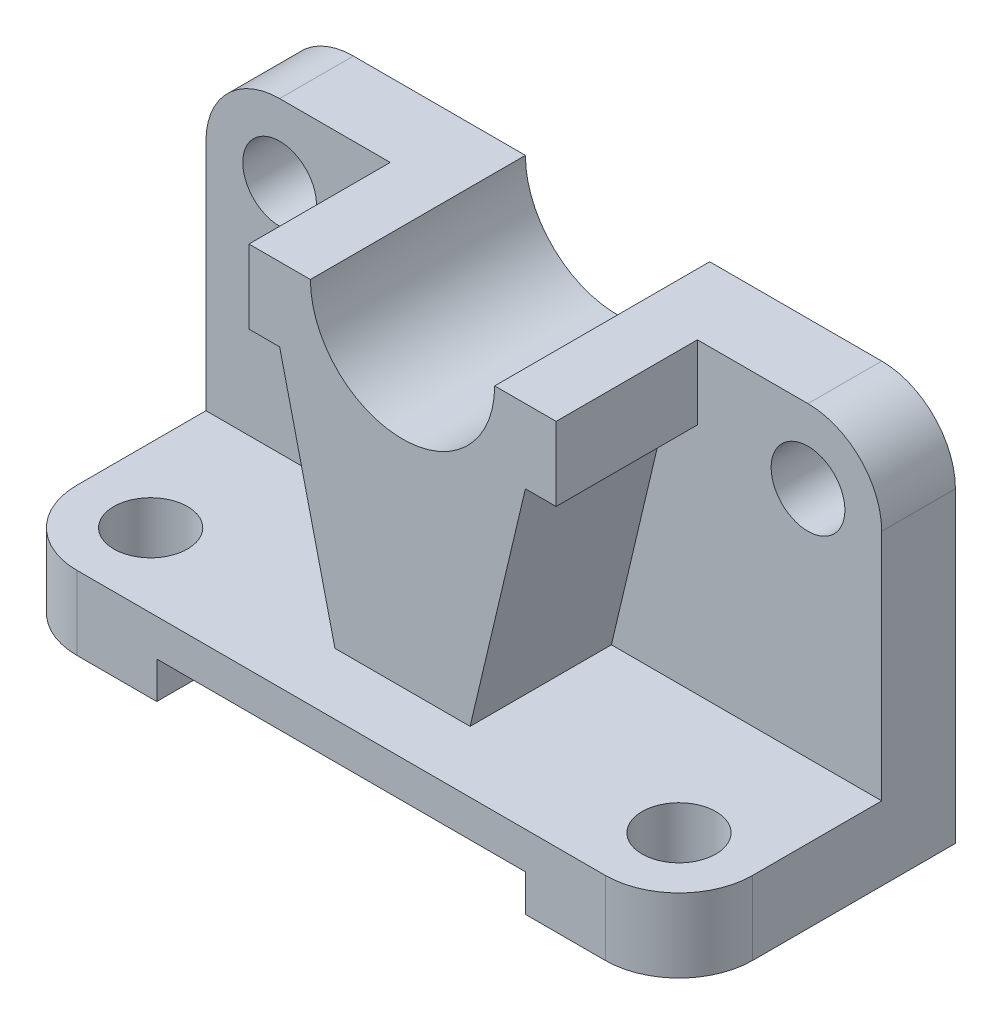
ISO-10303-21;
HEADER;
FILE_DESCRIPTION(('STEP AP214'),'2;1');
FILE_NAME('part.step','',(''),(''),'','','');
FILE_SCHEMA(('AUTOMOTIVE_DESIGN { 1 0 10303 214 1 1 1 1 }'));
ENDSEC;
DATA;
#1=APPLICATION_CONTEXT('core data for automotive mechanical design processes');
#2=APPLICATION_PROTOCOL_DEFINITION('international standard','automotive_design',2000,#1);
#3=PRODUCT_CONTEXT('',#1,'mechanical');
#4=PRODUCT('Part','Part','',(#3));
#5=PRODUCT_RELATED_PRODUCT_CATEGORY('part','',(#4));
#6=PRODUCT_DEFINITION_FORMATION('','',#4);
#7=PRODUCT_DEFINITION_CONTEXT('part definition',#1,'design');
#8=PRODUCT_DEFINITION('design','',#6,#7);
#9=PRODUCT_DEFINITION_SHAPE('','',#8);
#10=(LENGTH_UNIT() NAMED_UNIT(*) SI_UNIT(.MILLI.,.METRE.));
#11=(NAMED_UNIT(*) PLANE_ANGLE_UNIT() SI_UNIT($,.RADIAN.));
#12=(NAMED_UNIT(*) SI_UNIT($,.STERADIAN.) SOLID_ANGLE_UNIT());
#13=UNCERTAINTY_MEASURE_WITH_UNIT(LENGTH_MEASURE(1.E-05),#10,'distance_accuracy_value','');
#14=(GEOMETRIC_REPRESENTATION_CONTEXT(3) GLOBAL_UNCERTAINTY_ASSIGNED_CONTEXT((#13)) GLOBAL_UNIT_ASSIGNED_CONTEXT((#10,
#11,#12)) REPRESENTATION_CONTEXT('',''));
#15=CARTESIAN_POINT('',(0.,0.,0.));
#16=DIRECTION('',(0.,0.,1.));
#17=DIRECTION('',(1.,0.,0.));
#18=AXIS2_PLACEMENT_3D('',#15,#16,#17);
#19=CARTESIAN_POINT('',(43.,50.,-10.5));
#20=DIRECTION('',(0.,0.,1.));
#21=DIRECTION('',(1.,0.,0.));
#22=AXIS2_PLACEMENT_3D('',#19,#20,#21);
#23=PLANE('',#22);
#24=CARTESIAN_POINT('',(-43.,50.,-10.5));
#25=DIRECTION('',(0.,0.,-1.));
#26=DIRECTION('',(-1.,0.,0.));
#27=AXIS2_PLACEMENT_3D('',#24,#25,#26);
#28=CIRCLE('',#27,5.99999999999999);
#29=CARTESIAN_POINT('',(-49.,50.,-10.5));
#30=VERTEX_POINT('',#29);
#31=EDGE_CURVE('E298',#30,#30,#28,.T.);
#32=ORIENTED_EDGE('',*,*,#31,.T.);
#33=EDGE_LOOP('',(#32));
#34=FACE_BOUND('',#33,.T.);
#35=DIRECTION('',(1.,0.,0.));
#36=VECTOR('',#35,1.);
#37=CARTESIAN_POINT('',(-43.,12.,-10.5));
#38=LINE('',#37,#36);
#39=CARTESIAN_POINT('',(-55.,12.,-10.5));
#40=VERTEX_POINT('',#39);
#41=CARTESIAN_POINT('',(-11.,12.,-10.5));
#42=VERTEX_POINT('',#41);
#43=EDGE_CURVE('E347',#40,#42,#38,.T.);
#44=ORIENTED_EDGE('',*,*,#43,.T.);
#45=DIRECTION('',(0.230466383879213,-0.973080287490009,0.));
#46=VECTOR('',#45,1.);
#47=CARTESIAN_POINT('',(-7.72459016393442,-1.82950819672131,-10.5));
#48=LINE('',#47,#46);
#49=CARTESIAN_POINT('',(-20.,50.,-10.5));
#50=VERTEX_POINT('',#49);
#51=EDGE_CURVE('E245',#50,#42,#48,.T.);
#52=ORIENTED_EDGE('',*,*,#51,.F.);
#53=DIRECTION('',(-1.,0.,0.));
#54=VECTOR('',#53,1.);
#55=CARTESIAN_POINT('',(0.,50.,-10.5));
#56=LINE('',#55,#54);
#57=CARTESIAN_POINT('',(-25.,50.,-10.5));
#58=VERTEX_POINT('',#57);
#59=EDGE_CURVE('E250',#50,#58,#56,.T.);
#60=ORIENTED_EDGE('',*,*,#59,.T.);
#61=DIRECTION('',(0.,-1.,0.));
#62=VECTOR('',#61,1.);
#63=CARTESIAN_POINT('',(-25.,50.,-10.5));
#64=LINE('',#63,#62);
#65=CARTESIAN_POINT('',(-25.,62.,-10.5));
#66=VERTEX_POINT('',#65);
#67=EDGE_CURVE('E11',#66,#58,#64,.T.);
#68=ORIENTED_EDGE('',*,*,#67,.F.);
#69=DIRECTION('',(1.,0.,0.));
#70=VECTOR('',#69,1.);
#71=CARTESIAN_POINT('',(42.9999999999999,62.,-10.5));
#72=LINE('',#71,#70);
#73=CARTESIAN_POINT('',(-42.9999999999999,62.,-10.5));
#74=VERTEX_POINT('',#73);
#75=EDGE_CURVE('E321',#74,#66,#72,.T.);
#76=ORIENTED_EDGE('',*,*,#75,.F.);
#77=CARTESIAN_POINT('',(-43.,50.,-10.5));
#78=DIRECTION('',(0.,0.,-1.));
#79=DIRECTION('',(1.,0.,0.));
#80=AXIS2_PLACEMENT_3D('',#77,#78,#79);
#81=CIRCLE('',#80,12.);
#82=CARTESIAN_POINT('',(-55.,49.9999999999999,-10.5));
#83=VERTEX_POINT('',#82);
#84=EDGE_CURVE('E320',#83,#74,#81,.T.);
#85=ORIENTED_EDGE('',*,*,#84,.F.);
#86=DIRECTION('',(0.,1.,0.));
#87=VECTOR('',#86,1.);
#88=CARTESIAN_POINT('',(-55.,0.,-10.5));
#89=LINE('',#88,#87);
#90=EDGE_CURVE('E314',#40,#83,#89,.T.);
#91=ORIENTED_EDGE('',*,*,#90,.F.);
#92=EDGE_LOOP('',(#44,#52,#60,#68,#76,#85,#91));
#93=FACE_BOUND('',#92,.T.);
#94=ADVANCED_FACE('F50',(#34,#93),#23,.T.);
#95=DIRECTION('',(-0.230466383879213,-0.97308028749001,0.));
#96=VECTOR('',#95,1.);
#97=CARTESIAN_POINT('',(7.72459016393442,-1.82950819672131,-10.5));
#98=LINE('',#97,#96);
#99=CARTESIAN_POINT('',(20.,50.,-10.5));
#100=VERTEX_POINT('',#99);
#101=CARTESIAN_POINT('',(11.,12.,-10.5));
#102=VERTEX_POINT('',#101);
#103=EDGE_CURVE('E260',#100,#102,#98,.T.);
#104=ORIENTED_EDGE('',*,*,#103,.T.);
#105=CARTESIAN_POINT('',(55.,12.,-10.5));
#106=VERTEX_POINT('',#105);
#107=EDGE_CURVE('E339',#102,#106,#38,.T.);
#108=ORIENTED_EDGE('',*,*,#107,.T.);
#109=DIRECTION('',(0.,-1.,0.));
#110=VECTOR('',#109,1.);
#111=CARTESIAN_POINT('',(55.,0.,-10.5));
#112=LINE('',#111,#110);
#113=CARTESIAN_POINT('',(55.,49.9999999999999,-10.5));
#114=VERTEX_POINT('',#113);
#115=EDGE_CURVE('E313',#114,#106,#112,.T.);
#116=ORIENTED_EDGE('',*,*,#115,.F.);
#117=CARTESIAN_POINT('',(43.,50.,-10.5));
#118=DIRECTION('',(0.,0.,-1.));
#119=DIRECTION('',(1.,0.,0.));
#120=AXIS2_PLACEMENT_3D('',#117,#118,#119);
#121=CIRCLE('',#120,12.);
#122=CARTESIAN_POINT('',(42.9999999999999,62.,-10.5));
#123=VERTEX_POINT('',#122);
#124=EDGE_CURVE('E322',#123,#114,#121,.T.);
#125=ORIENTED_EDGE('',*,*,#124,.F.);
#126=CARTESIAN_POINT('',(25.,62.,-10.5));
#127=VERTEX_POINT('',#126);
#128=EDGE_CURVE('E319',#127,#123,#72,.T.);
#129=ORIENTED_EDGE('',*,*,#128,.F.);
#130=DIRECTION('',(0.,-1.,0.));
#131=VECTOR('',#130,1.);
#132=CARTESIAN_POINT('',(25.,50.,-10.5));
#133=LINE('',#132,#131);
#134=CARTESIAN_POINT('',(25.,50.,-10.5));
#135=VERTEX_POINT('',#134);
#136=EDGE_CURVE('E218',#127,#135,#133,.T.);
#137=ORIENTED_EDGE('',*,*,#136,.T.);
#138=DIRECTION('',(1.,0.,0.));
#139=VECTOR('',#138,1.);
#140=CARTESIAN_POINT('',(0.,50.,-10.5));
#141=LINE('',#140,#139);
#142=EDGE_CURVE('E62',#100,#135,#141,.T.);
#143=ORIENTED_EDGE('',*,*,#142,.F.);
#144=EDGE_LOOP('',(#104,#108,#116,#125,#129,#137,#143));
#145=FACE_BOUND('',#144,.T.);
#146=CARTESIAN_POINT('',(43.,50.,-10.5));
#147=DIRECTION('',(0.,0.,-1.));
#148=DIRECTION('',(-1.,0.,0.));
#149=AXIS2_PLACEMENT_3D('',#146,#147,#148);
#150=CIRCLE('',#149,5.99999999999999);
#151=CARTESIAN_POINT('',(37.,50.,-10.5));
#152=VERTEX_POINT('',#151);
#153=EDGE_CURVE('E304',#152,#152,#150,.T.);
#154=ORIENTED_EDGE('',*,*,#153,.T.);
#155=EDGE_LOOP('',(#154));
#156=FACE_BOUND('',#155,.T.);
#157=ADVANCED_FACE('F454',(#145,#156),#23,.T.);
#158=CARTESIAN_POINT('',(0.,62.,12.5));
#159=DIRECTION('',(0.,0.,-1.));
#160=DIRECTION('',(-1.,0.,0.));
#161=AXIS2_PLACEMENT_3D('',#158,#159,#160);
#162=PLANE('',#161);
#163=DIRECTION('',(1.,0.,0.));
#164=VECTOR('',#163,1.);
#165=CARTESIAN_POINT('',(0.,50.,12.5));
#166=LINE('',#165,#164);
#167=CARTESIAN_POINT('',(-25.,50.,12.5));
#168=VERTEX_POINT('',#167);
#169=CARTESIAN_POINT('',(-20.,50.,12.5));
#170=VERTEX_POINT('',#169);
#171=EDGE_CURVE('E253',#168,#170,#166,.T.);
#172=ORIENTED_EDGE('',*,*,#171,.T.);
#173=DIRECTION('',(-0.230466383879213,0.97308028749001,0.));
#174=VECTOR('',#173,1.);
#175=CARTESIAN_POINT('',(-7.72459016393442,-1.82950819672131,12.5));
#176=LINE('',#175,#174);
#177=CARTESIAN_POINT('',(-11.,12.,12.5));
#178=VERTEX_POINT('',#177);
#179=EDGE_CURVE('E251',#178,#170,#176,.T.);
#180=ORIENTED_EDGE('',*,*,#179,.F.);
#181=DIRECTION('',(1.,0.,0.));
#182=VECTOR('',#181,1.);
#183=CARTESIAN_POINT('',(0.,12.,12.5));
#184=LINE('',#183,#182);
#185=CARTESIAN_POINT('',(11.,12.,12.5));
#186=VERTEX_POINT('',#185);
#187=EDGE_CURVE('E227',#178,#186,#184,.T.);
#188=ORIENTED_EDGE('',*,*,#187,.T.);
#189=DIRECTION('',(0.230466383879213,0.973080287490009,0.));
#190=VECTOR('',#189,1.);
#191=CARTESIAN_POINT('',(7.72459016393442,-1.82950819672131,12.5));
#192=LINE('',#191,#190);
#193=CARTESIAN_POINT('',(20.,50.,12.5));
#194=VERTEX_POINT('',#193);
#195=EDGE_CURVE('E217',#186,#194,#192,.T.);
#196=ORIENTED_EDGE('',*,*,#195,.T.);
#197=DIRECTION('',(-1.,0.,0.));
#198=VECTOR('',#197,1.);
#199=CARTESIAN_POINT('',(0.,50.,12.5));
#200=LINE('',#199,#198);
#201=CARTESIAN_POINT('',(25.,50.,12.5));
#202=VERTEX_POINT('',#201);
#203=EDGE_CURVE('E211',#202,#194,#200,.T.);
#204=ORIENTED_EDGE('',*,*,#203,.F.);
#205=DIRECTION('',(0.,-1.,0.));
#206=VECTOR('',#205,1.);
#207=CARTESIAN_POINT('',(25.,0.,12.5));
#208=LINE('',#207,#206);
#209=CARTESIAN_POINT('',(25.,62.,12.5));
#210=VERTEX_POINT('',#209);
#211=EDGE_CURVE('E216',#210,#202,#208,.T.);
#212=ORIENTED_EDGE('',*,*,#211,.F.);
#213=DIRECTION('',(1.,0.,0.));
#214=VECTOR('',#213,1.);
#215=CARTESIAN_POINT('',(25.,62.,12.5));
#216=LINE('',#215,#214);
#217=CARTESIAN_POINT('',(15.,62.,12.5));
#218=VERTEX_POINT('',#217);
#219=EDGE_CURVE('E264',#218,#210,#216,.T.);
#220=ORIENTED_EDGE('',*,*,#219,.F.);
#221=CARTESIAN_POINT('',(0.,62.,12.5));
#222=DIRECTION('',(0.,0.,1.));
#223=DIRECTION('',(-1.,0.,0.));
#224=AXIS2_PLACEMENT_3D('',#221,#222,#223);
#225=CIRCLE('',#224,15.);
#226=CARTESIAN_POINT('',(-15.,62.,12.5));
#227=VERTEX_POINT('',#226);
#228=EDGE_CURVE('E249',#227,#218,#225,.T.);
#229=ORIENTED_EDGE('',*,*,#228,.F.);
#230=DIRECTION('',(1.,0.,0.));
#231=VECTOR('',#230,1.);
#232=CARTESIAN_POINT('',(-15.,62.,12.5));
#233=LINE('',#232,#231);
#234=CARTESIAN_POINT('',(-25.,62.,12.5));
#235=VERTEX_POINT('',#234);
#236=EDGE_CURVE('E270',#235,#227,#233,.T.);
#237=ORIENTED_EDGE('',*,*,#236,.F.);
#238=DIRECTION('',(0.,-1.,0.));
#239=VECTOR('',#238,1.);
#240=CARTESIAN_POINT('',(-25.,0.,12.5));
#241=LINE('',#240,#239);
#242=EDGE_CURVE('E230',#235,#168,#241,.T.);
#243=ORIENTED_EDGE('',*,*,#242,.T.);
#244=EDGE_LOOP('',(#172,#180,#188,#196,#204,#212,#220,#229,#237,#243));
#245=FACE_BOUND('',#244,.T.);
#246=ADVANCED_FACE('F213',(#245),#162,.F.);
#247=CARTESIAN_POINT('',(42.9999999999999,62.,-10.5));
#248=DIRECTION('',(0.,1.,0.));
#249=DIRECTION('',(0.,0.,1.));
#250=AXIS2_PLACEMENT_3D('',#247,#248,#249);
#251=PLANE('',#250);
#252=DIRECTION('',(0.,0.,-1.));
#253=VECTOR('',#252,1.);
#254=CARTESIAN_POINT('',(25.,62.,12.5));
#255=LINE('',#254,#253);
#256=EDGE_CURVE('E69',#210,#127,#255,.T.);
#257=ORIENTED_EDGE('',*,*,#256,.T.);
#258=ORIENTED_EDGE('',*,*,#128,.T.);
#259=DIRECTION('',(0.,0.,-1.));
#260=VECTOR('',#259,1.);
#261=CARTESIAN_POINT('',(42.9999999999999,62.,-10.5));
#262=LINE('',#261,#260);
#263=CARTESIAN_POINT('',(42.9999999999999,62.,-22.5));
#264=VERTEX_POINT('',#263);
#265=EDGE_CURVE('E338',#123,#264,#262,.T.);
#266=ORIENTED_EDGE('',*,*,#265,.T.);
#267=DIRECTION('',(1.,0.,0.));
#268=VECTOR('',#267,1.);
#269=CARTESIAN_POINT('',(42.9999999999999,62.,-22.5));
#270=LINE('',#269,#268);
#271=CARTESIAN_POINT('',(15.,62.,-22.5));
#272=VERTEX_POINT('',#271);
#273=EDGE_CURVE('E329',#272,#264,#270,.T.);
#274=ORIENTED_EDGE('',*,*,#273,.F.);
#275=DIRECTION('',(0.,0.,-1.));
#276=VECTOR('',#275,1.);
#277=CARTESIAN_POINT('',(15.,62.,57.5));
#278=LINE('',#277,#276);
#279=EDGE_CURVE('E276',#218,#272,#278,.T.);
#280=ORIENTED_EDGE('',*,*,#279,.F.);
#281=ORIENTED_EDGE('',*,*,#219,.T.);
#282=EDGE_LOOP('',(#257,#258,#266,#274,#280,#281));
#283=FACE_BOUND('',#282,.T.);
#284=ADVANCED_FACE('F444',(#283),#251,.T.);
#285=CARTESIAN_POINT('',(-43.,0.,10.5));
#286=DIRECTION('',(0.,1.,0.));
#287=DIRECTION('',(0.,0.,1.));
#288=AXIS2_PLACEMENT_3D('',#285,#286,#287);
#289=PLANE('',#288);
#290=CARTESIAN_POINT('',(-43.,0.,10.5));
#291=DIRECTION('',(0.,1.,0.));
#292=DIRECTION('',(0.,0.,1.));
#293=AXIS2_PLACEMENT_3D('',#290,#291,#292);
#294=CIRCLE('',#293,6.);
#295=CARTESIAN_POINT('',(-43.,0.,16.5));
#296=VERTEX_POINT('',#295);
#297=EDGE_CURVE('E354',#296,#296,#294,.T.);
#298=ORIENTED_EDGE('',*,*,#297,.T.);
#299=EDGE_LOOP('',(#298));
#300=FACE_BOUND('',#299,.T.);
#301=DIRECTION('',(-1.,0.,0.));
#302=VECTOR('',#301,1.);
#303=CARTESIAN_POINT('',(-55.,0.,-22.5));
#304=LINE('',#303,#302);
#305=CARTESIAN_POINT('',(-30.,0.,-22.5));
#306=VERTEX_POINT('',#305);
#307=CARTESIAN_POINT('',(-55.,0.,-22.5));
#308=VERTEX_POINT('',#307);
#309=EDGE_CURVE('E387',#306,#308,#304,.T.);
#310=ORIENTED_EDGE('',*,*,#309,.F.);
#311=DIRECTION('',(0.,0.,1.));
#312=VECTOR('',#311,1.);
#313=CARTESIAN_POINT('',(-30.,0.,-57.5));
#314=LINE('',#313,#312);
#315=CARTESIAN_POINT('',(-30.,0.,22.5));
#316=VERTEX_POINT('',#315);
#317=EDGE_CURVE('E287',#306,#316,#314,.T.);
#318=ORIENTED_EDGE('',*,*,#317,.T.);
#319=DIRECTION('',(1.,0.,0.));
#320=VECTOR('',#319,1.);
#321=CARTESIAN_POINT('',(-42.9999999999999,0.,22.5));
#322=LINE('',#321,#320);
#323=CARTESIAN_POINT('',(-42.9999999999999,0.,22.5));
#324=VERTEX_POINT('',#323);
#325=EDGE_CURVE('E377',#324,#316,#322,.T.);
#326=ORIENTED_EDGE('',*,*,#325,.F.);
#327=CARTESIAN_POINT('',(-43.,0.,10.5));
#328=DIRECTION('',(0.,1.,0.));
#329=DIRECTION('',(0.,0.,1.));
#330=AXIS2_PLACEMENT_3D('',#327,#328,#329);
#331=CIRCLE('',#330,12.);
#332=CARTESIAN_POINT('',(-55.,0.,10.4999999999999));
#333=VERTEX_POINT('',#332);
#334=EDGE_CURVE('E376',#333,#324,#331,.T.);
#335=ORIENTED_EDGE('',*,*,#334,.F.);
#336=DIRECTION('',(0.,0.,1.));
#337=VECTOR('',#336,1.);
#338=CARTESIAN_POINT('',(-55.,0.,-22.5));
#339=LINE('',#338,#337);
#340=EDGE_CURVE('E357',#308,#333,#339,.T.);
#341=ORIENTED_EDGE('',*,*,#340,.F.);
#342=EDGE_LOOP('',(#310,#318,#326,#335,#341));
#343=FACE_BOUND('',#342,.T.);
#344=ADVANCED_FACE('F423',(#300,#343),#289,.F.);
#345=CARTESIAN_POINT('',(-43.,12.,10.5));
#346=DIRECTION('',(0.,1.,0.));
#347=DIRECTION('',(0.,0.,1.));
#348=AXIS2_PLACEMENT_3D('',#345,#346,#347);
#349=PLANE('',#348);
#350=DIRECTION('',(0.,0.,1.));
#351=VECTOR('',#350,1.);
#352=CARTESIAN_POINT('',(11.,12.,-22.5));
#353=LINE('',#352,#351);
#354=EDGE_CURVE('E237',#102,#186,#353,.T.);
#355=ORIENTED_EDGE('',*,*,#354,.T.);
#356=ORIENTED_EDGE('',*,*,#187,.F.);
#357=DIRECTION('',(0.,0.,1.));
#358=VECTOR('',#357,1.);
#359=CARTESIAN_POINT('',(-11.,12.,-22.5));
#360=LINE('',#359,#358);
#361=EDGE_CURVE('E239',#42,#178,#360,.T.);
#362=ORIENTED_EDGE('',*,*,#361,.F.);
#363=ORIENTED_EDGE('',*,*,#43,.F.);
#364=DIRECTION('',(0.,0.,1.));
#365=VECTOR('',#364,1.);
#366=CARTESIAN_POINT('',(-55.,12.,-22.5));
#367=LINE('',#366,#365);
#368=CARTESIAN_POINT('',(-55.,12.,10.4999999999999));
#369=VERTEX_POINT('',#368);
#370=EDGE_CURVE('E362',#40,#369,#367,.T.);
#371=ORIENTED_EDGE('',*,*,#370,.T.);
#372=CARTESIAN_POINT('',(-43.,12.,10.5));
#373=DIRECTION('',(0.,1.,0.));
#374=DIRECTION('',(0.,0.,1.));
#375=AXIS2_PLACEMENT_3D('',#372,#373,#374);
#376=CIRCLE('',#375,12.);
#377=CARTESIAN_POINT('',(-42.9999999999999,12.,22.5));
#378=VERTEX_POINT('',#377);
#379=EDGE_CURVE('E365',#369,#378,#376,.T.);
#380=ORIENTED_EDGE('',*,*,#379,.T.);
#381=DIRECTION('',(1.,0.,0.));
#382=VECTOR('',#381,1.);
#383=CARTESIAN_POINT('',(-42.9999999999999,12.,22.5));
#384=LINE('',#383,#382);
#385=CARTESIAN_POINT('',(42.9999999999999,12.,22.5));
#386=VERTEX_POINT('',#385);
#387=EDGE_CURVE('E370',#378,#386,#384,.T.);
#388=ORIENTED_EDGE('',*,*,#387,.T.);
#389=CARTESIAN_POINT('',(43.,12.,10.5));
#390=DIRECTION('',(0.,1.,0.));
#391=DIRECTION('',(0.,0.,1.));
#392=AXIS2_PLACEMENT_3D('',#389,#390,#391);
#393=CIRCLE('',#392,12.);
#394=CARTESIAN_POINT('',(55.,12.,10.4999999999999));
#395=VERTEX_POINT('',#394);
#396=EDGE_CURVE('E369',#386,#395,#393,.T.);
#397=ORIENTED_EDGE('',*,*,#396,.T.);
#398=DIRECTION('',(0.,0.,-1.));
#399=VECTOR('',#398,1.);
#400=CARTESIAN_POINT('',(55.,12.,-22.5));
#401=LINE('',#400,#399);
#402=EDGE_CURVE('E371',#395,#106,#401,.T.);
#403=ORIENTED_EDGE('',*,*,#402,.T.);
#404=ORIENTED_EDGE('',*,*,#107,.F.);
#405=EDGE_LOOP('',(#355,#356,#362,#363,#371,#380,#388,#397,#403,#404));
#406=FACE_BOUND('',#405,.T.);
#407=CARTESIAN_POINT('',(-43.,12.,10.5));
#408=DIRECTION('',(0.,1.,0.));
#409=DIRECTION('',(0.,0.,1.));
#410=AXIS2_PLACEMENT_3D('',#407,#408,#409);
#411=CIRCLE('',#410,6.);
#412=CARTESIAN_POINT('',(-43.,12.,16.5));
#413=VERTEX_POINT('',#412);
#414=EDGE_CURVE('E356',#413,#413,#411,.T.);
#415=ORIENTED_EDGE('',*,*,#414,.F.);
#416=EDGE_LOOP('',(#415));
#417=FACE_BOUND('',#416,.T.);
#418=CARTESIAN_POINT('',(43.,12.,10.5));
#419=DIRECTION('',(0.,1.,0.));
#420=DIRECTION('',(0.,0.,1.));
#421=AXIS2_PLACEMENT_3D('',#418,#419,#420);
#422=CIRCLE('',#421,6.);
#423=CARTESIAN_POINT('',(43.,12.,16.5));
#424=VERTEX_POINT('',#423);
#425=EDGE_CURVE('E348',#424,#424,#422,.T.);
#426=ORIENTED_EDGE('',*,*,#425,.F.);
#427=EDGE_LOOP('',(#426));
#428=FACE_BOUND('',#427,.T.);
#429=ADVANCED_FACE('F458',(#406,#417,#428),#349,.T.);
#430=CARTESIAN_POINT('',(30.,0.,22.5));
#431=VERTEX_POINT('',#430);
#432=CARTESIAN_POINT('',(42.9999999999999,0.,22.5));
#433=VERTEX_POINT('',#432);
#434=EDGE_CURVE('E378',#431,#433,#322,.T.);
#435=ORIENTED_EDGE('',*,*,#434,.F.);
#436=DIRECTION('',(0.,0.,1.));
#437=VECTOR('',#436,1.);
#438=CARTESIAN_POINT('',(30.,0.,-57.5));
#439=LINE('',#438,#437);
#440=CARTESIAN_POINT('',(30.,0.,-22.5));
#441=VERTEX_POINT('',#440);
#442=EDGE_CURVE('E293',#441,#431,#439,.T.);
#443=ORIENTED_EDGE('',*,*,#442,.F.);
#444=CARTESIAN_POINT('',(55.,0.,-22.5));
#445=VERTEX_POINT('',#444);
#446=EDGE_CURVE('E364',#445,#441,#304,.T.);
#447=ORIENTED_EDGE('',*,*,#446,.F.);
#448=DIRECTION('',(0.,0.,-1.));
#449=VECTOR('',#448,1.);
#450=CARTESIAN_POINT('',(55.,0.,-22.5));
#451=LINE('',#450,#449);
#452=CARTESIAN_POINT('',(55.,0.,10.4999999999999));
#453=VERTEX_POINT('',#452);
#454=EDGE_CURVE('E383',#453,#445,#451,.T.);
#455=ORIENTED_EDGE('',*,*,#454,.F.);
#456=CARTESIAN_POINT('',(43.,0.,10.5));
#457=DIRECTION('',(0.,1.,0.));
#458=DIRECTION('',(0.,0.,1.));
#459=AXIS2_PLACEMENT_3D('',#456,#457,#458);
#460=CIRCLE('',#459,12.);
#461=EDGE_CURVE('E385',#433,#453,#460,.T.);
#462=ORIENTED_EDGE('',*,*,#461,.F.);
#463=EDGE_LOOP('',(#435,#443,#447,#455,#462));
#464=FACE_BOUND('',#463,.T.);
#465=CARTESIAN_POINT('',(43.,0.,10.5));
#466=DIRECTION('',(0.,1.,0.));
#467=DIRECTION('',(0.,0.,1.));
#468=AXIS2_PLACEMENT_3D('',#465,#466,#467);
#469=CIRCLE('',#468,6.);
#470=CARTESIAN_POINT('',(43.,0.,16.5));
#471=VERTEX_POINT('',#470);
#472=EDGE_CURVE('E349',#471,#471,#469,.T.);
#473=ORIENTED_EDGE('',*,*,#472,.T.);
#474=EDGE_LOOP('',(#473));
#475=FACE_BOUND('',#474,.T.);
#476=ADVANCED_FACE('F469',(#464,#475),#289,.F.);
#477=CARTESIAN_POINT('',(-55.,12.,-22.5));
#478=DIRECTION('',(1.,0.,0.));
#479=DIRECTION('',(0.,0.,-1.));
#480=AXIS2_PLACEMENT_3D('',#477,#478,#479);
#481=PLANE('',#480);
#482=ORIENTED_EDGE('',*,*,#370,.F.);
#483=ORIENTED_EDGE('',*,*,#90,.T.);
#484=DIRECTION('',(0.,0.,-1.));
#485=VECTOR('',#484,1.);
#486=CARTESIAN_POINT('',(-55.,49.9999999999999,-10.5));
#487=LINE('',#486,#485);
#488=CARTESIAN_POINT('',(-55.,49.9999999999999,-22.5));
#489=VERTEX_POINT('',#488);
#490=EDGE_CURVE('E330',#83,#489,#487,.T.);
#491=ORIENTED_EDGE('',*,*,#490,.T.);
#492=DIRECTION('',(0.,-1.,0.));
#493=VECTOR('',#492,1.);
#494=CARTESIAN_POINT('',(-55.,12.,-22.5));
#495=LINE('',#494,#493);
#496=EDGE_CURVE('E372',#489,#308,#495,.T.);
#497=ORIENTED_EDGE('',*,*,#496,.T.);
#498=ORIENTED_EDGE('',*,*,#340,.T.);
#499=DIRECTION('',(0.,-1.,0.));
#500=VECTOR('',#499,1.);
#501=CARTESIAN_POINT('',(-55.,12.,10.4999999999999));
#502=LINE('',#501,#500);
#503=EDGE_CURVE('E401',#369,#333,#502,.T.);
#504=ORIENTED_EDGE('',*,*,#503,.F.);
#505=EDGE_LOOP('',(#482,#483,#491,#497,#498,#504));
#506=FACE_BOUND('',#505,.T.);
#507=ADVANCED_FACE('F47',(#506),#481,.F.);
#508=CARTESIAN_POINT('',(-43.,12.,10.5));
#509=DIRECTION('',(0.,-1.,0.));
#510=DIRECTION('',(0.,0.,-1.));
#511=AXIS2_PLACEMENT_3D('',#508,#509,#510);
#512=CYLINDRICAL_SURFACE('',#511,12.);
#513=ORIENTED_EDGE('',*,*,#334,.T.);
#514=DIRECTION('',(0.,-1.,0.));
#515=VECTOR('',#514,1.);
#516=CARTESIAN_POINT('',(-42.9999999999999,12.,22.5));
#517=LINE('',#516,#515);
#518=EDGE_CURVE('E399',#378,#324,#517,.T.);
#519=ORIENTED_EDGE('',*,*,#518,.F.);
#520=ORIENTED_EDGE('',*,*,#379,.F.);
#521=ORIENTED_EDGE('',*,*,#503,.T.);
#522=EDGE_LOOP('',(#513,#519,#520,#521));
#523=FACE_BOUND('',#522,.T.);
#524=ADVANCED_FACE('F488',(#523),#512,.T.);
#525=CARTESIAN_POINT('',(-42.9999999999999,12.,22.5));
#526=DIRECTION('',(0.,0.,-1.));
#527=DIRECTION('',(-1.,0.,0.));
#528=AXIS2_PLACEMENT_3D('',#525,#526,#527);
#529=PLANE('',#528);
#530=ORIENTED_EDGE('',*,*,#325,.T.);
#531=DIRECTION('',(0.,-1.,0.));
#532=VECTOR('',#531,1.);
#533=CARTESIAN_POINT('',(-30.,0.,22.5));
#534=LINE('',#533,#532);
#535=CARTESIAN_POINT('',(-30.,6.,22.5));
#536=VERTEX_POINT('',#535);
#537=EDGE_CURVE('E281',#536,#316,#534,.T.);
#538=ORIENTED_EDGE('',*,*,#537,.F.);
#539=DIRECTION('',(-1.,0.,0.));
#540=VECTOR('',#539,1.);
#541=CARTESIAN_POINT('',(-30.,6.,22.5));
#542=LINE('',#541,#540);
#543=CARTESIAN_POINT('',(30.,6.,22.5));
#544=VERTEX_POINT('',#543);
#545=EDGE_CURVE('E286',#544,#536,#542,.T.);
#546=ORIENTED_EDGE('',*,*,#545,.F.);
#547=DIRECTION('',(0.,1.,0.));
#548=VECTOR('',#547,1.);
#549=CARTESIAN_POINT('',(30.,0.,22.5));
#550=LINE('',#549,#548);
#551=EDGE_CURVE('E284',#431,#544,#550,.T.);
#552=ORIENTED_EDGE('',*,*,#551,.F.);
#553=ORIENTED_EDGE('',*,*,#434,.T.);
#554=DIRECTION('',(0.,-1.,0.));
#555=VECTOR('',#554,1.);
#556=CARTESIAN_POINT('',(42.9999999999999,12.,22.5));
#557=LINE('',#556,#555);
#558=EDGE_CURVE('E400',#386,#433,#557,.T.);
#559=ORIENTED_EDGE('',*,*,#558,.F.);
#560=ORIENTED_EDGE('',*,*,#387,.F.);
#561=ORIENTED_EDGE('',*,*,#518,.T.);
#562=EDGE_LOOP('',(#530,#538,#546,#552,#553,#559,#560,#561));
#563=FACE_BOUND('',#562,.T.);
#564=ADVANCED_FACE('F485',(#563),#529,.F.);
#565=CARTESIAN_POINT('',(43.,12.,10.5));
#566=DIRECTION('',(0.,-1.,0.));
#567=DIRECTION('',(0.,0.,-1.));
#568=AXIS2_PLACEMENT_3D('',#565,#566,#567);
#569=CYLINDRICAL_SURFACE('',#568,12.);
#570=ORIENTED_EDGE('',*,*,#461,.T.);
#571=DIRECTION('',(0.,-1.,0.));
#572=VECTOR('',#571,1.);
#573=CARTESIAN_POINT('',(55.,12.,10.4999999999999));
#574=LINE('',#573,#572);
#575=EDGE_CURVE('E393',#395,#453,#574,.T.);
#576=ORIENTED_EDGE('',*,*,#575,.F.);
#577=ORIENTED_EDGE('',*,*,#396,.F.);
#578=ORIENTED_EDGE('',*,*,#558,.T.);
#579=EDGE_LOOP('',(#570,#576,#577,#578));
#580=FACE_BOUND('',#579,.T.);
#581=ADVANCED_FACE('F546',(#580),#569,.T.);
#582=CARTESIAN_POINT('',(55.,12.,-22.5));
#583=DIRECTION('',(-1.,0.,0.));
#584=DIRECTION('',(0.,0.,1.));
#585=AXIS2_PLACEMENT_3D('',#582,#583,#584);
#586=PLANE('',#585);
#587=ORIENTED_EDGE('',*,*,#454,.T.);
#588=DIRECTION('',(0.,-1.,0.));
#589=VECTOR('',#588,1.);
#590=CARTESIAN_POINT('',(55.,12.,-22.5));
#591=LINE('',#590,#589);
#592=CARTESIAN_POINT('',(55.,49.9999999999999,-22.5));
#593=VERTEX_POINT('',#592);
#594=EDGE_CURVE('E391',#593,#445,#591,.T.);
#595=ORIENTED_EDGE('',*,*,#594,.F.);
#596=DIRECTION('',(0.,0.,-1.));
#597=VECTOR('',#596,1.);
#598=CARTESIAN_POINT('',(55.,49.9999999999999,-10.5));
#599=LINE('',#598,#597);
#600=EDGE_CURVE('E333',#114,#593,#599,.T.);
#601=ORIENTED_EDGE('',*,*,#600,.F.);
#602=ORIENTED_EDGE('',*,*,#115,.T.);
#603=ORIENTED_EDGE('',*,*,#402,.F.);
#604=ORIENTED_EDGE('',*,*,#575,.T.);
#605=EDGE_LOOP('',(#587,#595,#601,#602,#603,#604));
#606=FACE_BOUND('',#605,.T.);
#607=ADVANCED_FACE('F455',(#606),#586,.F.);
#608=CARTESIAN_POINT('',(-55.,12.,-22.5));
#609=DIRECTION('',(0.,0.,1.));
#610=DIRECTION('',(1.,0.,0.));
#611=AXIS2_PLACEMENT_3D('',#608,#609,#610);
#612=PLANE('',#611);
#613=CARTESIAN_POINT('',(-42.9999999999999,62.,-22.5));
#614=VERTEX_POINT('',#613);
#615=CARTESIAN_POINT('',(-15.,62.,-22.5));
#616=VERTEX_POINT('',#615);
#617=EDGE_CURVE('E332',#614,#616,#270,.T.);
#618=ORIENTED_EDGE('',*,*,#617,.T.);
#619=CARTESIAN_POINT('',(0.,62.,-22.5));
#620=DIRECTION('',(0.,0.,-1.));
#621=DIRECTION('',(-1.,0.,0.));
#622=AXIS2_PLACEMENT_3D('',#619,#620,#621);
#623=CIRCLE('',#622,15.);
#624=EDGE_CURVE('E272',#272,#616,#623,.T.);
#625=ORIENTED_EDGE('',*,*,#624,.F.);
#626=ORIENTED_EDGE('',*,*,#273,.T.);
#627=CARTESIAN_POINT('',(43.,50.,-22.5));
#628=DIRECTION('',(0.,0.,-1.));
#629=DIRECTION('',(1.,0.,0.));
#630=AXIS2_PLACEMENT_3D('',#627,#628,#629);
#631=CIRCLE('',#630,12.);
#632=EDGE_CURVE('E312',#264,#593,#631,.T.);
#633=ORIENTED_EDGE('',*,*,#632,.T.);
#634=ORIENTED_EDGE('',*,*,#594,.T.);
#635=ORIENTED_EDGE('',*,*,#446,.T.);
#636=DIRECTION('',(0.,1.,0.));
#637=VECTOR('',#636,1.);
#638=CARTESIAN_POINT('',(30.,12.,-22.5));
#639=LINE('',#638,#637);
#640=CARTESIAN_POINT('',(30.,6.,-22.5));
#641=VERTEX_POINT('',#640);
#642=EDGE_CURVE('E406',#441,#641,#639,.T.);
#643=ORIENTED_EDGE('',*,*,#642,.T.);
#644=DIRECTION('',(-1.,0.,0.));
#645=VECTOR('',#644,1.);
#646=CARTESIAN_POINT('',(-55.,6.,-22.5));
#647=LINE('',#646,#645);
#648=CARTESIAN_POINT('',(-30.,6.,-22.5));
#649=VERTEX_POINT('',#648);
#650=EDGE_CURVE('E408',#641,#649,#647,.T.);
#651=ORIENTED_EDGE('',*,*,#650,.T.);
#652=DIRECTION('',(0.,-1.,0.));
#653=VECTOR('',#652,1.);
#654=CARTESIAN_POINT('',(-30.,12.,-22.5));
#655=LINE('',#654,#653);
#656=EDGE_CURVE('E54',#649,#306,#655,.T.);
#657=ORIENTED_EDGE('',*,*,#656,.T.);
#658=ORIENTED_EDGE('',*,*,#309,.T.);
#659=ORIENTED_EDGE('',*,*,#496,.F.);
#660=CARTESIAN_POINT('',(-43.,50.,-22.5));
#661=DIRECTION('',(0.,0.,-1.));
#662=DIRECTION('',(1.,0.,0.));
#663=AXIS2_PLACEMENT_3D('',#660,#661,#662);
#664=CIRCLE('',#663,12.);
#665=EDGE_CURVE('E306',#489,#614,#664,.T.);
#666=ORIENTED_EDGE('',*,*,#665,.T.);
#667=EDGE_LOOP('',(#618,#625,#626,#633,#634,#635,#643,#651,#657,#658,#659,#666));
#668=FACE_BOUND('',#667,.T.);
#669=CARTESIAN_POINT('',(-43.,50.,-22.5));
#670=DIRECTION('',(0.,0.,-1.));
#671=DIRECTION('',(-1.,0.,0.));
#672=AXIS2_PLACEMENT_3D('',#669,#670,#671);
#673=CIRCLE('',#672,5.99999999999999);
#674=CARTESIAN_POINT('',(-49.,50.,-22.5));
#675=VERTEX_POINT('',#674);
#676=EDGE_CURVE('E295',#675,#675,#673,.T.);
#677=ORIENTED_EDGE('',*,*,#676,.F.);
#678=EDGE_LOOP('',(#677));
#679=FACE_BOUND('',#678,.T.);
#680=CARTESIAN_POINT('',(43.,50.,-22.5));
#681=DIRECTION('',(0.,0.,-1.));
#682=DIRECTION('',(-1.,0.,0.));
#683=AXIS2_PLACEMENT_3D('',#680,#681,#682);
#684=CIRCLE('',#683,5.99999999999999);
#685=CARTESIAN_POINT('',(37.,50.,-22.5));
#686=VERTEX_POINT('',#685);
#687=EDGE_CURVE('E305',#686,#686,#684,.T.);
#688=ORIENTED_EDGE('',*,*,#687,.F.);
#689=EDGE_LOOP('',(#688));
#690=FACE_BOUND('',#689,.T.);
#691=ADVANCED_FACE('F412',(#668,#679,#690),#612,.F.);
#692=CARTESIAN_POINT('',(-43.,12.,10.5));
#693=DIRECTION('',(0.,-1.,0.));
#694=DIRECTION('',(0.,0.,-1.));
#695=AXIS2_PLACEMENT_3D('',#692,#693,#694);
#696=CYLINDRICAL_SURFACE('',#695,6.);
#697=ORIENTED_EDGE('',*,*,#414,.T.);
#698=EDGE_LOOP('',(#697));
#699=FACE_BOUND('',#698,.T.);
#700=ORIENTED_EDGE('',*,*,#297,.F.);
#701=EDGE_LOOP('',(#700));
#702=FACE_BOUND('',#701,.T.);
#703=ADVANCED_FACE('F531',(#699,#702),#696,.F.);
#704=CARTESIAN_POINT('',(43.,12.,10.5));
#705=DIRECTION('',(0.,-1.,0.));
#706=DIRECTION('',(0.,0.,-1.));
#707=AXIS2_PLACEMENT_3D('',#704,#705,#706);
#708=CYLINDRICAL_SURFACE('',#707,6.);
#709=ORIENTED_EDGE('',*,*,#425,.T.);
#710=EDGE_LOOP('',(#709));
#711=FACE_BOUND('',#710,.T.);
#712=ORIENTED_EDGE('',*,*,#472,.F.);
#713=EDGE_LOOP('',(#712));
#714=FACE_BOUND('',#713,.T.);
#715=ADVANCED_FACE('F527',(#711,#714),#708,.F.);
#716=CARTESIAN_POINT('',(43.,50.,-10.5));
#717=DIRECTION('',(0.,0.,-1.));
#718=DIRECTION('',(-1.,0.,0.));
#719=AXIS2_PLACEMENT_3D('',#716,#717,#718);
#720=CYLINDRICAL_SURFACE('',#719,12.);
#721=ORIENTED_EDGE('',*,*,#632,.F.);
#722=ORIENTED_EDGE('',*,*,#265,.F.);
#723=ORIENTED_EDGE('',*,*,#124,.T.);
#724=ORIENTED_EDGE('',*,*,#600,.T.);
#725=EDGE_LOOP('',(#721,#722,#723,#724));
#726=FACE_BOUND('',#725,.T.);
#727=ADVANCED_FACE('F448',(#726),#720,.T.);
#728=ORIENTED_EDGE('',*,*,#75,.T.);
#729=DIRECTION('',(0.,0.,-1.));
#730=VECTOR('',#729,1.);
#731=CARTESIAN_POINT('',(-25.,62.,12.5));
#732=LINE('',#731,#730);
#733=EDGE_CURVE('E269',#235,#66,#732,.T.);
#734=ORIENTED_EDGE('',*,*,#733,.F.);
#735=ORIENTED_EDGE('',*,*,#236,.T.);
#736=DIRECTION('',(0.,0.,-1.));
#737=VECTOR('',#736,1.);
#738=CARTESIAN_POINT('',(-15.,62.,57.5));
#739=LINE('',#738,#737);
#740=EDGE_CURVE('E280',#616,#227,#739,.F.);
#741=ORIENTED_EDGE('',*,*,#740,.F.);
#742=ORIENTED_EDGE('',*,*,#617,.F.);
#743=DIRECTION('',(0.,0.,-1.));
#744=VECTOR('',#743,1.);
#745=CARTESIAN_POINT('',(-42.9999999999999,62.,-10.5));
#746=LINE('',#745,#744);
#747=EDGE_CURVE('E345',#74,#614,#746,.T.);
#748=ORIENTED_EDGE('',*,*,#747,.F.);
#749=EDGE_LOOP('',(#728,#734,#735,#741,#742,#748));
#750=FACE_BOUND('',#749,.T.);
#751=ADVANCED_FACE('F440',(#750),#251,.T.);
#752=CARTESIAN_POINT('',(-43.,50.,-10.5));
#753=DIRECTION('',(0.,0.,-1.));
#754=DIRECTION('',(-1.,0.,0.));
#755=AXIS2_PLACEMENT_3D('',#752,#753,#754);
#756=CYLINDRICAL_SURFACE('',#755,12.);
#757=ORIENTED_EDGE('',*,*,#665,.F.);
#758=ORIENTED_EDGE('',*,*,#490,.F.);
#759=ORIENTED_EDGE('',*,*,#84,.T.);
#760=ORIENTED_EDGE('',*,*,#747,.T.);
#761=EDGE_LOOP('',(#757,#758,#759,#760));
#762=FACE_BOUND('',#761,.T.);
#763=ADVANCED_FACE('F435',(#762),#756,.T.);
#764=CARTESIAN_POINT('',(43.,50.,-10.5));
#765=DIRECTION('',(0.,0.,-1.));
#766=DIRECTION('',(-1.,0.,0.));
#767=AXIS2_PLACEMENT_3D('',#764,#765,#766);
#768=CYLINDRICAL_SURFACE('',#767,5.99999999999999);
#769=ORIENTED_EDGE('',*,*,#153,.F.);
#770=EDGE_LOOP('',(#769));
#771=FACE_BOUND('',#770,.T.);
#772=ORIENTED_EDGE('',*,*,#687,.T.);
#773=EDGE_LOOP('',(#772));
#774=FACE_BOUND('',#773,.T.);
#775=ADVANCED_FACE('F523',(#771,#774),#768,.F.);
#776=CARTESIAN_POINT('',(-43.,50.,-10.5));
#777=DIRECTION('',(0.,0.,-1.));
#778=DIRECTION('',(-1.,0.,0.));
#779=AXIS2_PLACEMENT_3D('',#776,#777,#778);
#780=CYLINDRICAL_SURFACE('',#779,5.99999999999999);
#781=ORIENTED_EDGE('',*,*,#31,.F.);
#782=EDGE_LOOP('',(#781));
#783=FACE_BOUND('',#782,.T.);
#784=ORIENTED_EDGE('',*,*,#676,.T.);
#785=EDGE_LOOP('',(#784));
#786=FACE_BOUND('',#785,.T.);
#787=ADVANCED_FACE('F590',(#783,#786),#780,.F.);
#788=CARTESIAN_POINT('',(-30.,0.,-57.5));
#789=DIRECTION('',(-1.,0.,0.));
#790=DIRECTION('',(0.,0.,1.));
#791=AXIS2_PLACEMENT_3D('',#788,#789,#790);
#792=PLANE('',#791);
#793=DIRECTION('',(0.,0.,1.));
#794=VECTOR('',#793,1.);
#795=CARTESIAN_POINT('',(-30.,6.,-57.5));
#796=LINE('',#795,#794);
#797=EDGE_CURVE('E289',#649,#536,#796,.T.);
#798=ORIENTED_EDGE('',*,*,#797,.T.);
#799=ORIENTED_EDGE('',*,*,#537,.T.);
#800=ORIENTED_EDGE('',*,*,#317,.F.);
#801=ORIENTED_EDGE('',*,*,#656,.F.);
#802=EDGE_LOOP('',(#798,#799,#800,#801));
#803=FACE_BOUND('',#802,.T.);
#804=ADVANCED_FACE('F477',(#803),#792,.F.);
#805=CARTESIAN_POINT('',(-30.,6.,-57.5));
#806=DIRECTION('',(0.,1.,0.));
#807=DIRECTION('',(0.,0.,1.));
#808=AXIS2_PLACEMENT_3D('',#805,#806,#807);
#809=PLANE('',#808);
#810=DIRECTION('',(0.,0.,1.));
#811=VECTOR('',#810,1.);
#812=CARTESIAN_POINT('',(30.,6.,-57.5));
#813=LINE('',#812,#811);
#814=EDGE_CURVE('E291',#641,#544,#813,.T.);
#815=ORIENTED_EDGE('',*,*,#814,.T.);
#816=ORIENTED_EDGE('',*,*,#545,.T.);
#817=ORIENTED_EDGE('',*,*,#797,.F.);
#818=ORIENTED_EDGE('',*,*,#650,.F.);
#819=EDGE_LOOP('',(#815,#816,#817,#818));
#820=FACE_BOUND('',#819,.T.);
#821=ADVANCED_FACE('F476',(#820),#809,.F.);
#822=CARTESIAN_POINT('',(30.,0.,-57.5));
#823=DIRECTION('',(1.,0.,0.));
#824=DIRECTION('',(0.,0.,-1.));
#825=AXIS2_PLACEMENT_3D('',#822,#823,#824);
#826=PLANE('',#825);
#827=ORIENTED_EDGE('',*,*,#442,.T.);
#828=ORIENTED_EDGE('',*,*,#551,.T.);
#829=ORIENTED_EDGE('',*,*,#814,.F.);
#830=ORIENTED_EDGE('',*,*,#642,.F.);
#831=EDGE_LOOP('',(#827,#828,#829,#830));
#832=FACE_BOUND('',#831,.T.);
#833=ADVANCED_FACE('F475',(#832),#826,.F.);
#834=CARTESIAN_POINT('',(0.,62.,57.5));
#835=DIRECTION('',(0.,0.,-1.));
#836=DIRECTION('',(-1.,0.,0.));
#837=AXIS2_PLACEMENT_3D('',#834,#835,#836);
#838=CYLINDRICAL_SURFACE('',#837,15.);
#839=ORIENTED_EDGE('',*,*,#279,.T.);
#840=ORIENTED_EDGE('',*,*,#624,.T.);
#841=ORIENTED_EDGE('',*,*,#740,.T.);
#842=ORIENTED_EDGE('',*,*,#228,.T.);
#843=EDGE_LOOP('',(#839,#840,#841,#842));
#844=FACE_BOUND('',#843,.T.);
#845=ADVANCED_FACE('F442',(#844),#838,.F.);
#846=CARTESIAN_POINT('',(7.72459016393442,-1.82950819672131,-15.6744554471111));
#847=DIRECTION('',(0.973080287490009,-0.230466383879213,0.));
#848=DIRECTION('',(0.230466383879213,0.97308028749001,0.));
#849=AXIS2_PLACEMENT_3D('',#846,#847,#848);
#850=PLANE('',#849);
#851=DIRECTION('',(0.,0.,1.));
#852=VECTOR('',#851,1.);
#853=CARTESIAN_POINT('',(20.,50.,-15.6744554471111));
#854=LINE('',#853,#852);
#855=EDGE_CURVE('E256',#100,#194,#854,.T.);
#856=ORIENTED_EDGE('',*,*,#855,.T.);
#857=ORIENTED_EDGE('',*,*,#195,.F.);
#858=ORIENTED_EDGE('',*,*,#354,.F.);
#859=ORIENTED_EDGE('',*,*,#103,.F.);
#860=EDGE_LOOP('',(#856,#857,#858,#859));
#861=FACE_BOUND('',#860,.T.);
#862=ADVANCED_FACE('F504',(#861),#850,.T.);
#863=CARTESIAN_POINT('',(0.,50.,-15.6744554471111));
#864=DIRECTION('',(0.,1.,0.));
#865=DIRECTION('',(0.,0.,1.));
#866=AXIS2_PLACEMENT_3D('',#863,#864,#865);
#867=PLANE('',#866);
#868=ORIENTED_EDGE('',*,*,#142,.T.);
#869=DIRECTION('',(0.,0.,1.));
#870=VECTOR('',#869,1.);
#871=CARTESIAN_POINT('',(25.,50.,-22.5));
#872=LINE('',#871,#870);
#873=EDGE_CURVE('E225',#135,#202,#872,.T.);
#874=ORIENTED_EDGE('',*,*,#873,.T.);
#875=ORIENTED_EDGE('',*,*,#203,.T.);
#876=ORIENTED_EDGE('',*,*,#855,.F.);
#877=EDGE_LOOP('',(#868,#874,#875,#876));
#878=FACE_BOUND('',#877,.T.);
#879=ADVANCED_FACE('F224',(#878),#867,.F.);
#880=CARTESIAN_POINT('',(0.,50.,-15.6744554471111));
#881=DIRECTION('',(0.,-1.,0.));
#882=DIRECTION('',(0.,0.,-1.));
#883=AXIS2_PLACEMENT_3D('',#880,#881,#882);
#884=PLANE('',#883);
#885=DIRECTION('',(0.,0.,1.));
#886=VECTOR('',#885,1.);
#887=CARTESIAN_POINT('',(-20.,50.,-15.6744554471111));
#888=LINE('',#887,#886);
#889=EDGE_CURVE('E248',#50,#170,#888,.T.);
#890=ORIENTED_EDGE('',*,*,#889,.T.);
#891=ORIENTED_EDGE('',*,*,#171,.F.);
#892=DIRECTION('',(0.,0.,1.));
#893=VECTOR('',#892,1.);
#894=CARTESIAN_POINT('',(-25.,50.,-22.5));
#895=LINE('',#894,#893);
#896=EDGE_CURVE('E226',#58,#168,#895,.T.);
#897=ORIENTED_EDGE('',*,*,#896,.F.);
#898=ORIENTED_EDGE('',*,*,#59,.F.);
#899=EDGE_LOOP('',(#890,#891,#897,#898));
#900=FACE_BOUND('',#899,.T.);
#901=ADVANCED_FACE('F500',(#900),#884,.T.);
#902=CARTESIAN_POINT('',(-7.72459016393442,-1.82950819672131,-15.6744554471111));
#903=DIRECTION('',(0.973080287490009,0.230466383879213,0.));
#904=DIRECTION('',(-0.230466383879213,0.973080287490009,0.));
#905=AXIS2_PLACEMENT_3D('',#902,#903,#904);
#906=PLANE('',#905);
#907=ORIENTED_EDGE('',*,*,#51,.T.);
#908=ORIENTED_EDGE('',*,*,#361,.T.);
#909=ORIENTED_EDGE('',*,*,#179,.T.);
#910=ORIENTED_EDGE('',*,*,#889,.F.);
#911=EDGE_LOOP('',(#907,#908,#909,#910));
#912=FACE_BOUND('',#911,.T.);
#913=ADVANCED_FACE('F498',(#912),#906,.F.);
#914=CARTESIAN_POINT('',(25.,0.,-22.5));
#915=DIRECTION('',(-1.,0.,0.));
#916=DIRECTION('',(0.,0.,1.));
#917=AXIS2_PLACEMENT_3D('',#914,#915,#916);
#918=PLANE('',#917);
#919=ORIENTED_EDGE('',*,*,#136,.F.);
#920=ORIENTED_EDGE('',*,*,#256,.F.);
#921=ORIENTED_EDGE('',*,*,#211,.T.);
#922=ORIENTED_EDGE('',*,*,#873,.F.);
#923=EDGE_LOOP('',(#919,#920,#921,#922));
#924=FACE_BOUND('',#923,.T.);
#925=ADVANCED_FACE('F228',(#924),#918,.F.);
#926=CARTESIAN_POINT('',(-25.,0.,-22.5));
#927=DIRECTION('',(-1.,0.,0.));
#928=DIRECTION('',(0.,0.,1.));
#929=AXIS2_PLACEMENT_3D('',#926,#927,#928);
#930=PLANE('',#929);
#931=ORIENTED_EDGE('',*,*,#733,.T.);
#932=ORIENTED_EDGE('',*,*,#67,.T.);
#933=ORIENTED_EDGE('',*,*,#896,.T.);
#934=ORIENTED_EDGE('',*,*,#242,.F.);
#935=EDGE_LOOP('',(#931,#932,#933,#934));
#936=FACE_BOUND('',#935,.T.);
#937=ADVANCED_FACE('F493',(#936),#930,.T.);
#938=CLOSED_SHELL('',(#94,#157,#246,#284,#344,#429,#476,#507,#524,#564,#581,#607,#691,#703,#715,
#727,#751,#763,#775,#787,#804,#821,#833,#845,#862,#879,#901,#913,#925,#937));
#939=MANIFOLD_SOLID_BREP('B2',#938);
#940=ADVANCED_BREP_SHAPE_REPRESENTATION('',(#18,#939),#14);
#941=SHAPE_DEFINITION_REPRESENTATION(#9,#940);
ENDSEC;
END-ISO-10303-21;
